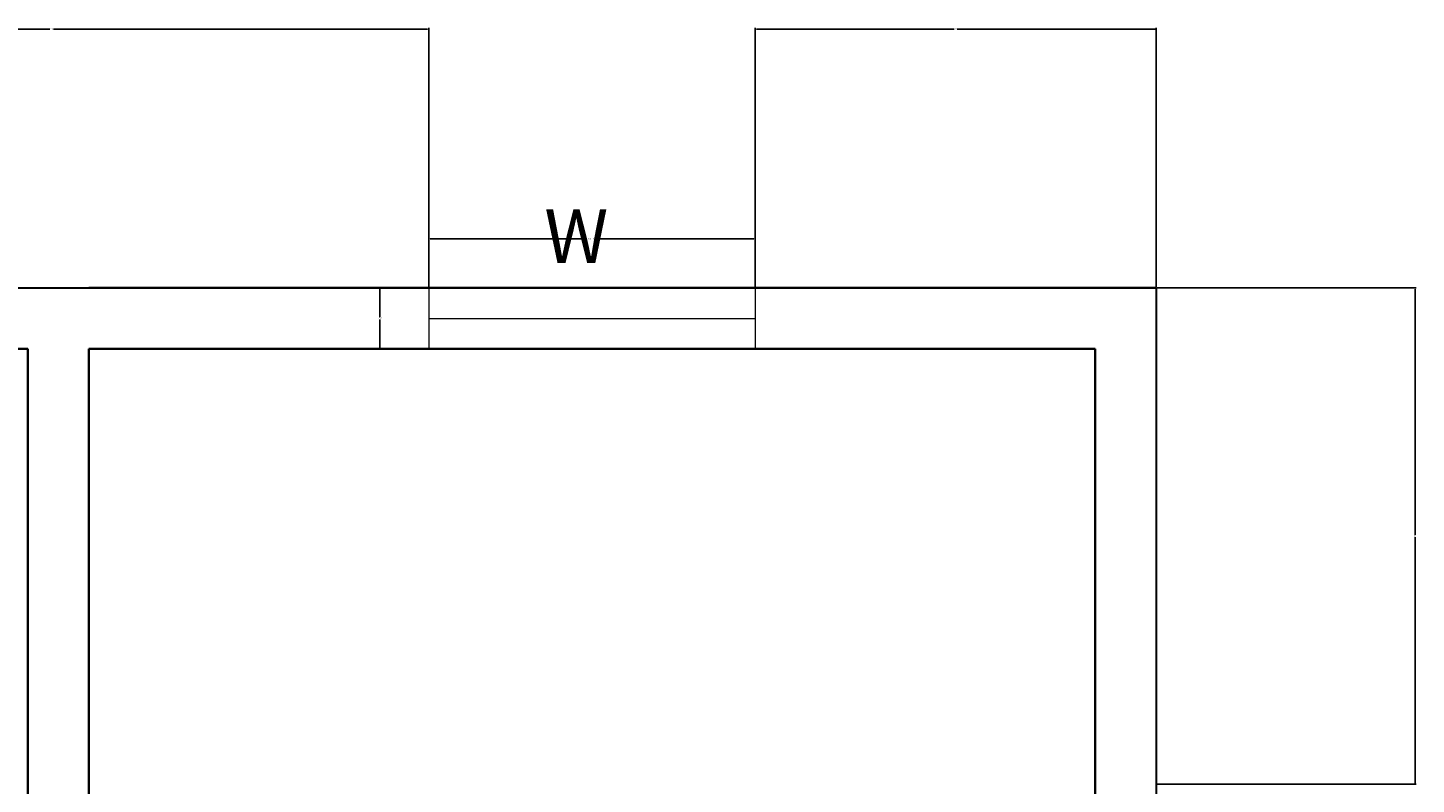
# Model space of a CAD drawing. Units: feet. Extents: x 2219 to 3039, y 1768 to 2369.
# Tile 16 of 16: x 2834 to 3039, y 2258 to 2369. Entities that reach past the tile are written whole.
import ezdxf

# ---------------------------------------------------------------- set-up
doc = ezdxf.new("R2010")
doc.units = ezdxf.units.FT
for name, color, linetype, lineweight in [('A-ANNO-DIMS', 2, 'Continuous', 18), ('A-ANNO-TEXT', 7, 'Continuous', 18), ('A-GLAZ', 4, 'Continuous', 18), ('A-WALL', 7, 'Continuous', 35), ('C-PROP', 7, 'Continuous', 30)]:
    doc.layers.add(name, color=color, linetype=linetype, lineweight=lineweight)
doc.styles.get("Standard").update_dxf_attribs({"font": 'arial.ttf'})
doc.dimstyles.get("Standard").update_dxf_attribs({"dimtxt": 0.18, "dimasz": 0.18, "dimexe": 0.18, "dimexo": 0.0625, "dimgap": 0.09, "dimtad": 0, "dimtih": 1, "dimtoh": 1, "dimdec": 4, "dimzin": 0, "dimdsep": 46, "dimtxsty": 'Standard', "dimcen": 0.09, "dimadec": 0, "dimazin": 0, "dimtfac": 1, "dimtdec": 4, "dimtofl": 0, "dimtmove": 0, "dimatfit": 3, "dimfxl": 1, "dimtolj": 1, "dimtzin": 0, "dimarcsym": 0})

# ---------------------------------------------------------------- blocks, each defined once
blk = doc.blocks.new('WINDOW-48')
for p, q in [((0, 9), (0, 0)), ((48, 9), (48, 0)), ((0, 4.5), (48, 4.5))]:
    blk.add_line(p, q)
blk = doc.blocks.new('*D34')
at = {"layer": 'A-ANNO-DIMS', "color": 0, "lineweight": -2, "transparency": 16777216}
for p, q in [((2893.4, 2330.99), (2893.4, 2338.3)), ((2893.58, 2338.12), (2916.28, 2338.12)), ((2941.22, 2338.12), (2918.52, 2338.12)), ((2941.4, 2330.99), (2941.4, 2338.3))]:
    blk.add_line(p, q, dxfattribs=at)
at = {"layer": 'A-ANNO-DIMS', "color": 0, "transparency": 16777216}
for points in [[(2893.58, 2338.15), (2893.58, 2338.09), (2893.4, 2338.12)], [(2941.22, 2338.15), (2941.22, 2338.09), (2941.4, 2338.12)]]:
    blk.add_solid(points, dxfattribs=at)
at = {"layer": 'Defpoints', "color": 0, "transparency": 16777216}
for p in [(2941.4, 2338.12), (2893.4, 2330.92), (2941.4, 2330.92)]:
    blk.add_point(p, dxfattribs=at)
at = {"layer": 'A-ANNO-DIMS', "color": 0, "transparency": 16777216, "insert": (2917.4, 2338.12), "char_height": 0.18, "attachment_point": 5}
blk.add_mtext('\\A1;WINDOW 48 TYP.', dxfattribs=at)
blk = doc.blocks.new('*D35')
at = {"layer": 'A-ANNO-DIMS', "color": 0, "lineweight": -2, "transparency": 16777216}
for p, q in [((2893.34, 2330.92), (2886.02, 2330.92)), ((2886.2, 2330.74), (2886.2, 2326.6)), ((2886.2, 2322.1), (2886.2, 2326.24)), ((2893.34, 2321.92), (2886.02, 2321.92))]:
    blk.add_line(p, q, dxfattribs=at)
at = {"layer": 'A-ANNO-DIMS', "color": 0, "transparency": 16777216}
for points in [[(2886.17, 2330.74), (2886.23, 2330.74), (2886.2, 2330.92)], [(2886.17, 2322.1), (2886.23, 2322.1), (2886.2, 2321.92)]]:
    blk.add_solid(points, dxfattribs=at)
at = {"layer": 'Defpoints', "color": 0, "transparency": 16777216}
for p in [(2886.2, 2330.92), (2893.4, 2330.92), (2893.4, 2321.92)]:
    blk.add_point(p, dxfattribs=at)
at = {"layer": 'A-ANNO-DIMS', "color": 0, "transparency": 16777216, "insert": (2886.2, 2326.42), "char_height": 0.18, "attachment_point": 5}
blk.add_mtext('\\A1;9 TYP.', dxfattribs=at)
blk = doc.blocks.new('*D51')
at = {"layer": 'A-ANNO-DIMS', "color": 0, "lineweight": -2, "transparency": 16777216}
for p, q in [((3000.46, 2330.92), (3038.63, 2330.92)), ((3038.45, 2330.74), (3038.45, 2294.6)), ((3038.45, 2258.1), (3038.45, 2294.24)), ((3000.46, 2257.92), (3038.63, 2257.92))]:
    blk.add_line(p, q, dxfattribs=at)
at = {"layer": 'A-ANNO-DIMS', "color": 0, "transparency": 16777216}
for points in [[(3038.42, 2330.74), (3038.48, 2330.74), (3038.45, 2330.92)], [(3038.42, 2258.1), (3038.48, 2258.1), (3038.45, 2257.92)]]:
    blk.add_solid(points, dxfattribs=at)
at = {"layer": 'Defpoints', "color": 0, "transparency": 16777216}
for p in [(3000.4, 2330.92), (3038.45, 2330.92), (3000.4, 2257.92)]:
    blk.add_point(p, dxfattribs=at)
at = {"layer": 'A-ANNO-DIMS', "color": 0, "transparency": 16777216, "insert": (3038.45, 2294.42), "char_height": 0.18, "attachment_point": 5}
blk.add_mtext('\\A1;73', dxfattribs=at)
blk = doc.blocks.new('*D57')
at = {"layer": 'A-ANNO-DIMS', "color": 0, "lineweight": -2, "transparency": 16777216}
for p, q in [((2782.4, 2330.99), (2782.4, 2369.15)), ((2893.4, 2330.99), (2893.4, 2369.15)), ((2782.58, 2368.97), (2837.64, 2368.97)), ((2893.22, 2368.97), (2838.16, 2368.97))]:
    blk.add_line(p, q, dxfattribs=at)
at = {"layer": 'A-ANNO-DIMS', "color": 0, "transparency": 16777216}
for points in [[(2782.58, 2369), (2782.58, 2368.94), (2782.4, 2368.97)], [(2893.22, 2369), (2893.22, 2368.94), (2893.4, 2368.97)]]:
    blk.add_solid(points, dxfattribs=at)
at = {"layer": 'Defpoints', "color": 0, "transparency": 16777216}
for p in [(2893.4, 2368.97), (2782.4, 2330.92), (2893.4, 2330.92)]:
    blk.add_point(p, dxfattribs=at)
at = {"layer": 'A-ANNO-DIMS', "color": 0, "transparency": 16777216, "insert": (2837.9, 2368.97), "char_height": 0.18, "attachment_point": 5}
blk.add_mtext('\\A1;111', dxfattribs=at)
blk = doc.blocks.new('*D58')
at = {"layer": 'A-ANNO-DIMS', "color": 0, "lineweight": -2, "transparency": 16777216}
for p, q in [((2941.4, 2330.99), (2941.4, 2369.15)), ((3000.4, 2330.99), (3000.4, 2369.15)), ((2941.58, 2368.97), (2970.68, 2368.97)), ((3000.22, 2368.97), (2971.12, 2368.97))]:
    blk.add_line(p, q, dxfattribs=at)
at = {"layer": 'A-ANNO-DIMS', "color": 0, "transparency": 16777216}
for points in [[(2941.58, 2369), (2941.58, 2368.94), (2941.4, 2368.97)], [(3000.22, 2369), (3000.22, 2368.94), (3000.4, 2368.97)]]:
    blk.add_solid(points, dxfattribs=at)
at = {"layer": 'Defpoints', "color": 0, "transparency": 16777216}
for p in [(3000.4, 2368.97), (2941.4, 2330.92), (3000.4, 2330.92)]:
    blk.add_point(p, dxfattribs=at)
at = {"layer": 'A-ANNO-DIMS', "color": 0, "transparency": 16777216, "insert": (2970.9, 2368.97), "char_height": 0.18, "attachment_point": 5}
blk.add_mtext('\\A1;59', dxfattribs=at)

msp = doc.modelspace()

# ---------------------------------------------------------------- linework, layer by layer
at = {"layer": 'A-WALL'}
for p, q in [((2843.4, 2330.923), (3000.4, 2330.923)), ((2610.4, 2321.923), (2834.4, 2321.923)), ((2834.4, 2321.923), (2834.4, 2204.687)), ((2843.4, 2321.923), (2843.4, 2204.687)), ((2843.4, 2321.923), (2991.4, 2321.923)), ((2991.4, 2321.923), (2991.4, 2121.923))]:
    msp.add_line(p, q, dxfattribs=at)
at = {"layer": 'C-PROP'}
for p, q in [((2314.4, 2330.923), (3000.4, 2330.923)), ((3000.4, 2330.923), (3000.4, 1828.923))]:
    msp.add_line(p, q, dxfattribs=at)

# ---------------------------------------------------------------- block references
at = {"layer": 'A-GLAZ'}
msp.add_blockref('WINDOW-48', (2893.4, 2321.923), dxfattribs=at)

# ---------------------------------------------------------------- texts
at = {"layer": 'A-ANNO-TEXT'}
msp.add_text('W', height=7.858, dxfattribs=at).set_placement((2910.378, 2334.574))

# ---------------------------------------------------------------- dimensions: what is measured, and where the dimension line sits
at = {"layer": 'A-ANNO-DIMS'}
for base, p1, p2, picture, middle in [((2893.4, 2368.973), (2782.4, 2330.923), (2893.4, 2330.923), '*D57', (2837.9, 2368.973)), ((3000.4, 2368.973), (2941.4, 2330.923), (3000.4, 2330.923), '*D58', (2970.9, 2368.973))]:
    dim = msp.add_linear_dim(base=base, p1=p1, p2=p2, dimstyle='Standard', override={"dimdec": 0, "dimlfac": 1, "dimrnd": 0, "dimzin": 0, "dimdsep": 46, "dimlunit": 2}, dxfattribs=at)
    dim.commit()
    dim.dimension.update_dxf_attribs({"geometry": picture, "text_midpoint": middle})
dim = msp.add_linear_dim(base=(2941.4, 2338.123), p1=(2893.4, 2330.923), p2=(2941.4, 2330.923), text='WINDOW <> TYP.', dimstyle='Standard', override={"dimdec": 0, "dimlfac": 1, "dimrnd": 0, "dimzin": 0, "dimdsep": 46, "dimlunit": 2}, dxfattribs=at)
dim.commit()
dim.dimension.update_dxf_attribs({"geometry": '*D34', "text_midpoint": (2917.4, 2338.123)})
dim = msp.add_linear_dim(base=(2886.2, 2330.923), p1=(2893.4, 2321.923), p2=(2893.4, 2330.923), angle=90, text='<> TYP.', dimstyle='Standard', override={"dimdec": 0, "dimlfac": 1, "dimrnd": 0, "dimzin": 0, "dimdsep": 46, "dimlunit": 2}, dxfattribs=at)
dim.commit()
dim.dimension.update_dxf_attribs({"geometry": '*D35', "text_midpoint": (2886.2, 2326.423)})
dim = msp.add_linear_dim(base=(3038.45, 2330.923), p1=(3000.4, 2257.923), p2=(3000.4, 2330.923), angle=90, dimstyle='Standard', override={"dimdec": 0, "dimlfac": 1, "dimrnd": 0, "dimzin": 0, "dimdsep": 46, "dimlunit": 2}, dxfattribs=at)
dim.commit()
dim.dimension.update_dxf_attribs({"geometry": '*D51', "text_midpoint": (3038.45, 2294.423)})

doc.saveas('drawing.dxf')
